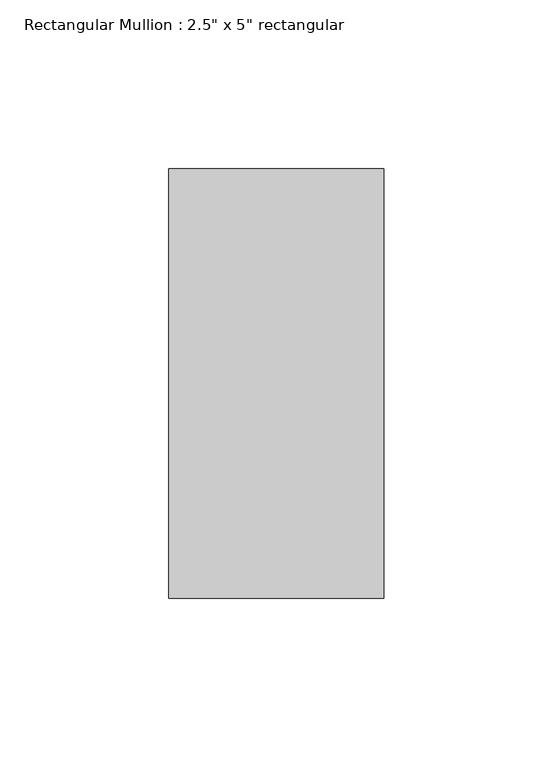
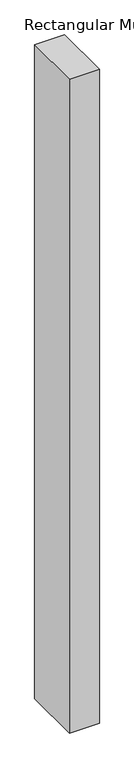
"""IFC4 building model written with IfcOpenShell, lengths in millimetres: member geometry."""

from ifc_helpers import new_model, si_unit, frame, origin, place, context, project, spatial, polyline, outline, extrude, source, transform, mapped, element, save


def member_64030597(model_context):
    return source(origin(), model_context, "Body", "SweptSolid", [
        extrude(outline(polyline([(0.0, 63.5), (0.0, -63.5), (-63.5, -63.5), (-63.5, 63.5), (0.0, 63.5)])), frame((0.0, 0.0, -1463.1285226), z_axis=(0.0, 0.0, 1.0), x_axis=(1.0, 0.0, 0.0)), (0.0, 0.0, 1.0), 1463.1285226),
    ])


if __name__ == "__main__":
    model = new_model("IFC4")
    model_context = context("Model", 3, world=origin())
    ifc_project = project(units=[si_unit("LENGTHUNIT", "METRE", prefix="MILLI")], contexts=[model_context])
    site = spatial("IfcSite", under=ifc_project)
    building = spatial("IfcBuilding", under=site)
    placement = place(None, origin())
    member_shape = member_64030597(model_context)
    element("IfcMember", 1, ObjectType="Rectangular Mullion : 2.5\" x 5\" rectangular", at=placement, inside=building, context=model_context, shape_type="MappedRepresentation", body=[
        mapped(member_shape, transform((0.0, 0.0, 0.0), x_axis=(1.0, 0.0, 0.0), y_axis=(0.0, 1.0, 0.0), z_axis=(0.0, 0.0, 1.0))),
    ])
    save(model, "model.ifc")

# Revit data of these elements
# Type "Rectangular Mullion : 2.5\" x 5\" rectangular"
#   built-in parameter 1007304 = 0.416667 (stored number, unit not read)
#   built-in parameter 1007301 = 0.104167 (stored number, unit not read)
#   built-in parameter 1007300 = 0.104167 (stored number, unit not read)
